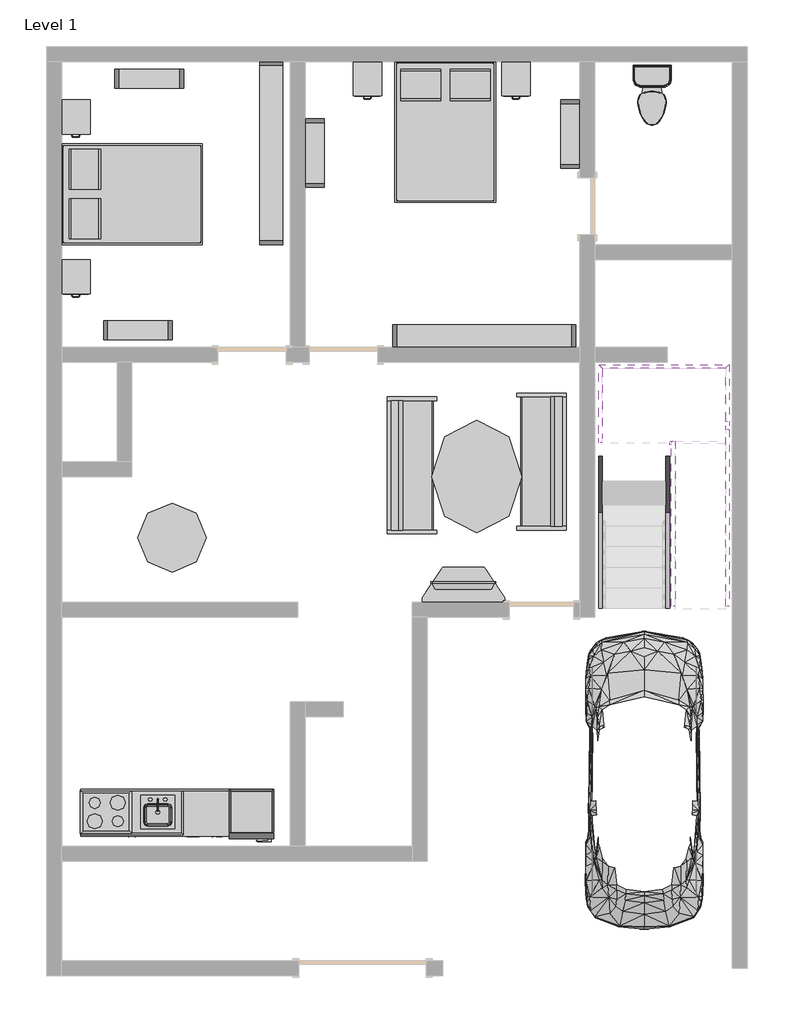
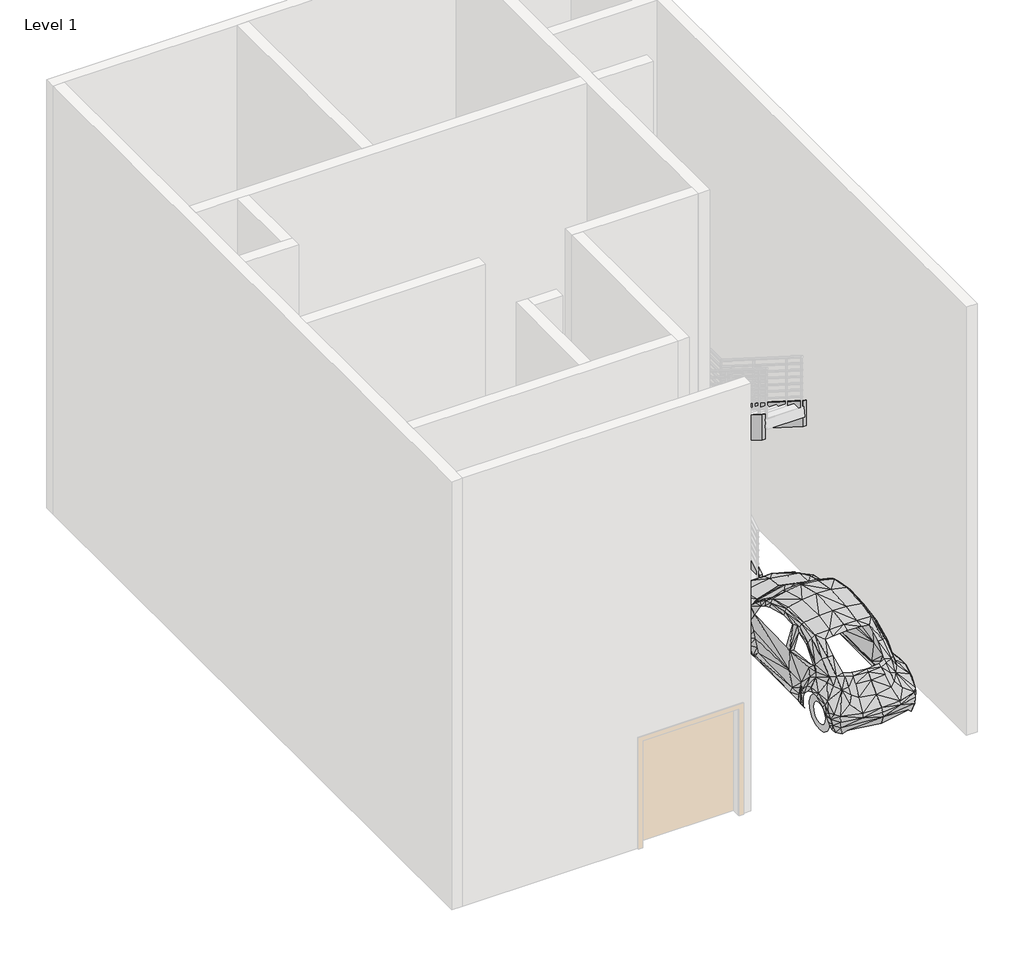
# One storey, part 4 of 4: 19 furniture elements, 8 members, 5 proxies, 2 flow terminals.
"""IFC4 building model written with IfcOpenShell, lengths in millimetres."""

from ifc_helpers import new_model, si_unit, frame, origin, place, context, project, spatial, polyline, outline, extrude, faceted_brep, transform, mapped, element, save
from components import m_cook_top_4_unit2_0615_x_500mm_249f3515, m_dishwasher_610_x_610_x_875mm_54ecfc4c, m_kitchenette_medium_1372mm_e05c6bec, m_rpc_beetle_m_rpc_beetle_b6d71803, m_refrigerator_600_x_660mm_a466bf94, m_sink_kitchen_island_450_x_450mm_f969cf2d, m_toilet_domestic_3d_m_toilet_domestic_3d_5cb52bd4, m_toilet_domestic_3d_m_toilet_domestic_3d_183bbd19, furniture_40ec15d9, furniture_0810mm_56245f3a, m_bed_box_1346_x_1880mm_double_b32eb57e, m_cabinet_file_2_drawer_0380_x_0457mm_9eec7cff, m_counter_top_w_sink_hole_600mm_depth_0a237b63, m_shelving_0915_x_0254_x_1830mm_1d5e155e, m_shelving_2440_x_0305_x_2134mm_59c1a9e4, m_sofa_1830mm_f9e8a66b, m_table_dining_round_w_chairs_0915mm_diameter_5defa876, m_table_ellipse_1500_x_1200mm_3917c766

model = new_model("IFC4")

# Units and contexts
model_context = context("Model", 3, world=origin())
ifc_project = project(units=[si_unit("LENGTHUNIT", "METRE", prefix="MILLI")], contexts=[model_context])

# Site, building, storey
site = spatial("IfcSite", under=ifc_project)
building = spatial("IfcBuilding", under=site)
storey = spatial("IfcBuildingStorey", under=building, Name="Level 1", Elevation=0.0)

# Proxies
placement = place(None, origin())
m_cook_top_4_unit2_0615_x_500mm_shape = m_cook_top_4_unit2_0615_x_500mm_249f3515(model_context)
element("IfcBuildingElementProxy", 1, Name="M_Cook Top-4 Unit2 : 0615 x 500mm", ObjectType="M_Cook Top-4 Unit2 : 0615 x 500mm", at=placement, inside=storey, context=model_context, shape_type="MappedRepresentation", body=[
    mapped(m_cook_top_4_unit2_0615_x_500mm_shape, transform((-6984.8389075, 2403.4805518, 0.0), x_axis=(1.0, 0.0, 0.0), y_axis=(0.0, 1.0, 0.0), z_axis=(0.0, 0.0, 1.0))),
])
m_dishwasher_610_x_610_x_875mm_shape = m_dishwasher_610_x_610_x_875mm_54ecfc4c(model_context)
element("IfcBuildingElementProxy", 2, Name="M_Dishwasher : 610 x 610 x 875mm", ObjectType="M_Dishwasher : 610 x 610 x 875mm", at=placement, inside=storey, context=model_context, shape_type="MappedRepresentation", body=[
    mapped(m_dishwasher_610_x_610_x_875mm_shape, transform((-6035.356376, 2136.830987, 0.0), x_axis=(1.0, 0.0, 0.0), y_axis=(0.0, 1.0, 0.0), z_axis=(0.0, 0.0, 1.0))),
])
m_kitchenette_medium_1372mm_shape = m_kitchenette_medium_1372mm_e05c6bec(model_context)
element("IfcBuildingElementProxy", 3, Name="M_Kitchenette - Medium : 1372mm", ObjectType="M_Kitchenette - Medium : 1372mm", at=placement, inside=storey, context=model_context, shape_type="MappedRepresentation", body=[
    mapped(m_kitchenette_medium_1372mm_shape, transform((-6660.5766124, 2708.4805518, 0.0), x_axis=(1.0, 0.0, 0.0), y_axis=(0.0, 1.0, 0.0), z_axis=(0.0, 0.0, 1.0))),
])
m_rpc_beetle_m_rpc_beetle_shape = m_rpc_beetle_m_rpc_beetle_b6d71803(model_context)
element("IfcBuildingElementProxy", 4, Name="M_RPC Beetle : M_RPC Beetle", ObjectType="M_RPC Beetle : M_RPC Beetle", at=placement, inside=storey, context=model_context, shape_type="MappedRepresentation", body=[
    mapped(m_rpc_beetle_m_rpc_beetle_shape, transform((192.3610925, 1592.0805518, 0.0), x_axis=(1.0, 0.0, 0.0), y_axis=(0.0, 1.0, 0.0), z_axis=(0.0, 0.0, 1.0))),
])
m_refrigerator_600_x_660mm_shape = m_refrigerator_600_x_660mm_a466bf94(model_context)
element("IfcBuildingElementProxy", 5, Name="M_Refrigerator : 600 x 660mm", ObjectType="M_Refrigerator : 600 x 660mm", at=placement, inside=storey, context=model_context, shape_type="MappedRepresentation", body=[
    mapped(m_refrigerator_600_x_660mm_shape, transform((-4994.0377648, 2412.2654616, 0.0), x_axis=(1.0, 0.0, 0.0), y_axis=(0.0, 1.0, 0.0), z_axis=(0.0, 0.0, 1.0))),
])

# Flow terminals
m_sink_kitchen_island_450_x_450mm_shape = m_sink_kitchen_island_450_x_450mm_f969cf2d(model_context)
element("IfcFlowTerminal", 6, ObjectType="M_Sink Kitchen-Island : 450 x 450mm", at=placement, inside=storey, context=model_context, shape_type="MappedRepresentation", body=[
    mapped(m_sink_kitchen_island_450_x_450mm_shape, transform((-6314.528148, 2401.1351507, 0.0), x_axis=(1.0, 0.0, 0.0), y_axis=(0.0, 1.0, 0.0), z_axis=(0.0, 0.0, 1.0))),
])
m_toilet_domestic_3d_m_toilet_domestic_3d_shape = m_toilet_domestic_3d_m_toilet_domestic_3d_5cb52bd4(model_context)
m_toilet_domestic_3d_m_toilet_domestic_3d_2_shape = m_toilet_domestic_3d_m_toilet_domestic_3d_183bbd19(model_context)
element("IfcFlowTerminal", 7, ObjectType="M_Toilet-Domestic-3D : M_Toilet-Domestic-3D", at=placement, inside=storey, context=model_context, shape_type="MappedRepresentation", body=[
    mapped(m_toilet_domestic_3d_m_toilet_domestic_3d_shape, transform((294.5650652, 11866.9845245, 0.0), x_axis=(1.0, 0.0, 0.0), y_axis=(0.0, 1.0, 0.0), z_axis=(0.0, 0.0, 1.0))),
    mapped(m_toilet_domestic_3d_m_toilet_domestic_3d_2_shape, transform((294.5650652, 11866.9845245, 0.0), x_axis=(1.0, 0.0, 0.0), y_axis=(0.0, 1.0, 0.0), z_axis=(0.0, 0.0, 1.0))),
])

# Furniture
furniture_shape = furniture_40ec15d9(model_context)
element("IfcFurniture", 8, at=placement, inside=storey, context=model_context, shape_type="MappedRepresentation", body=[
    mapped(furniture_shape, transform((-2345.8269095, 5670.4805518, 0.0), x_axis=(1.0, 0.0, 0.0), y_axis=(0.0, 1.0, 0.0), z_axis=(0.0, 0.0, 1.0))),
])
furniture_0810mm_shape = furniture_0810mm_56245f3a(model_context)
element("IfcFurniture", 9, ObjectType="0810mm", at=placement, inside=storey, context=model_context, shape_type="MappedRepresentation", body=[
    mapped(furniture_0810mm_shape, transform((-2224.5834216, 5406.0718602, 0.0), x_axis=(-1.0000000000000002, 0.0, 0.0), y_axis=(0.0, -1.0000000000000002, 0.0), z_axis=(0.0, 0.0, 1.0))),
])
m_bed_box_1346_x_1880mm_double_shape = m_bed_box_1346_x_1880mm_double_b32eb57e(model_context)
element("IfcFurniture", 10, ObjectType="M_Bed-Box : 1346 x 1880mm - Double", at=placement, inside=storey, context=model_context, shape_type="MappedRepresentation", body=[
    mapped(m_bed_box_1346_x_1880mm_double_shape, transform((-6876.0684157, 10306.3280928, 0.0), x_axis=(0.0, 1.0000000000000002, 0.0), y_axis=(-1.0000000000000002, 0.0, 0.0), z_axis=(0.0, 0.0, 1.0))),
])
element("IfcFurniture", 11, ObjectType="M_Bed-Box : 1346 x 1880mm - Double", at=placement, inside=storey, context=model_context, shape_type="MappedRepresentation", body=[
    mapped(m_bed_box_1346_x_1880mm_double_shape, transform((-2800.9913665, 11708.51006, 0.0), x_axis=(1.0000000000000009, 0.0, 0.0), y_axis=(0.0, 1.0000000000000009, 0.0), z_axis=(0.0, 0.0, 1.0))),
])
m_cabinet_file_2_drawer_0380_x_0457mm_shape = m_cabinet_file_2_drawer_0380_x_0457mm_9eec7cff(model_context)
element("IfcFurniture", 12, ObjectType="M_Cabinet-File 2 Drawer : 0380 x 0457mm", at=placement, inside=storey, context=model_context, shape_type="MappedRepresentation", body=[
    mapped(m_cabinet_file_2_drawer_0380_x_0457mm_shape, transform((-3374.9424604, 12327.7148519, 0.0), x_axis=(1.0, 0.0, 0.0), y_axis=(0.0, 1.0, 0.0), z_axis=(0.0, 0.0, 1.0))),
])
element("IfcFurniture", 13, ObjectType="M_Cabinet-File 2 Drawer : 0380 x 0457mm", at=placement, inside=storey, context=model_context, shape_type="MappedRepresentation", body=[
    mapped(m_cabinet_file_2_drawer_0380_x_0457mm_shape, transform((-1393.7424604, 12327.7148519, 0.0), x_axis=(1.0, 0.0, 0.0), y_axis=(0.0, 1.0, 0.0), z_axis=(0.0, 0.0, 1.0))),
])
element("IfcFurniture", 14, ObjectType="M_Cabinet-File 2 Drawer : 0380 x 0457mm", at=placement, inside=storey, context=model_context, shape_type="MappedRepresentation", body=[
    mapped(m_cabinet_file_2_drawer_0380_x_0457mm_shape, transform((-7263.7424604, 11818.1148519, 0.0), x_axis=(1.0, 0.0, 0.0), y_axis=(0.0, 1.0, 0.0), z_axis=(0.0, 0.0, 1.0))),
])
element("IfcFurniture", 15, ObjectType="M_Cabinet-File 2 Drawer : 0380 x 0457mm", at=placement, inside=storey, context=model_context, shape_type="MappedRepresentation", body=[
    mapped(m_cabinet_file_2_drawer_0380_x_0457mm_shape, transform((-7263.7424604, 9686.1148519, 0.0), x_axis=(1.0, 0.0, 0.0), y_axis=(0.0, 1.0, 0.0), z_axis=(0.0, 0.0, 1.0))),
])
m_counter_top_w_sink_hole_600mm_depth_shape = m_counter_top_w_sink_hole_600mm_depth_0a237b63(model_context)
element("IfcFurniture", 16, ObjectType="M_Counter Top w Sink Hole : 600mm Depth", at=placement, inside=storey, context=model_context, shape_type="MappedRepresentation", body=[
    mapped(m_counter_top_w_sink_hole_600mm_depth_shape, transform((-6127.3766124, 2708.4805518, 0.0), x_axis=(1.0, 0.0, 0.0), y_axis=(0.0, 1.0, 0.0), z_axis=(0.0, 0.0, 1.0))),
])
m_shelving_0915_x_0254_x_1830mm_shape = m_shelving_0915_x_0254_x_1830mm_1d5e155e(model_context)
element("IfcFurniture", 17, ObjectType="M_Shelving : 0915 x 0254 x 1830mm", at=placement, inside=storey, context=model_context, shape_type="MappedRepresentation", body=[
    mapped(m_shelving_0915_x_0254_x_1830mm_shape, transform((-6411.9389075, 12490.3805518, 0.0), x_axis=(1.0, 0.0, 0.0), y_axis=(0.0, 1.0, 0.0), z_axis=(0.0, 0.0, 1.0))),
])
element("IfcFurniture", 18, ObjectType="M_Shelving : 0915 x 0254 x 1830mm", at=placement, inside=storey, context=model_context, shape_type="MappedRepresentation", body=[
    mapped(m_shelving_0915_x_0254_x_1830mm_shape, transform((-6564.3389075, 9135.8805518, 0.0), x_axis=(1.0, 0.0, 0.0), y_axis=(0.0, 1.0, 0.0), z_axis=(0.0, 0.0, 1.0))),
])
element("IfcFurniture", 19, ObjectType="M_Shelving : 0915 x 0254 x 1830mm", at=placement, inside=storey, context=model_context, shape_type="MappedRepresentation", body=[
    mapped(m_shelving_0915_x_0254_x_1830mm_shape, transform((-4508.2389075, 11192.4805518, 0.0), x_axis=(0.0, 1.0, 0.0), y_axis=(-1.0, 0.0, 0.0), z_axis=(0.0, 0.0, 1.0))),
])
element("IfcFurniture", 20, ObjectType="M_Shelving : 0915 x 0254 x 1830mm", at=placement, inside=storey, context=model_context, shape_type="MappedRepresentation", body=[
    mapped(m_shelving_0915_x_0254_x_1830mm_shape, transform((-1101.4389075, 11446.9805518, 0.0), x_axis=(0.0, 1.0, 0.0), y_axis=(-1.0, 0.0, 0.0), z_axis=(0.0, 0.0, 1.0))),
])
m_shelving_2440_x_0305_x_2134mm_shape = m_shelving_2440_x_0305_x_2134mm_59c1a9e4(model_context)
element("IfcFurniture", 21, ObjectType="M_Shelving : 2440 x 0305 x 2134mm", at=placement, inside=storey, context=model_context, shape_type="MappedRepresentation", body=[
    mapped(m_shelving_2440_x_0305_x_2134mm_shape, transform((-1942.0389075, 9058.1805518, 0.0), x_axis=(1.0, 0.0, 0.0), y_axis=(0.0, 1.0, 0.0), z_axis=(0.0, 0.0, 1.0))),
])
element("IfcFurniture", 22, ObjectType="M_Shelving : 2440 x 0305 x 2134mm", at=placement, inside=storey, context=model_context, shape_type="MappedRepresentation", body=[
    mapped(m_shelving_2440_x_0305_x_2134mm_shape, transform((-5090.7389075, 11192.4805518, 0.0), x_axis=(0.0, 1.0000000000000002, 0.0), y_axis=(-1.0000000000000002, 0.0, 0.0), z_axis=(0.0, 0.0, 1.0))),
])
m_sofa_1830mm_shape = m_sofa_1830mm_f9e8a66b(model_context)
element("IfcFurniture", 23, ObjectType="M_Sofa : 1830mm", at=placement, inside=storey, context=model_context, shape_type="MappedRepresentation", body=[
    mapped(m_sofa_1830mm_shape, transform((-1325.3930058, 7147.2510436, 0.0), x_axis=(0.0, -1.0000000000000007, 0.0), y_axis=(1.0000000000000007, 0.0, 0.0), z_axis=(0.0, 0.0, 1.0))),
])
element("IfcFurniture", 24, ObjectType="M_Sofa : 1830mm", at=placement, inside=storey, context=model_context, shape_type="MappedRepresentation", body=[
    mapped(m_sofa_1830mm_shape, transform((-2758.6848091, 6957.31006, 0.0), x_axis=(0.0, 1.0000000000000002, 0.0), y_axis=(-1.0000000000000002, 0.0, 0.0), z_axis=(0.0, 0.0, 1.0))),
])
m_table_dining_round_w_chairs_0915mm_diameter_shape = m_table_dining_round_w_chairs_0915mm_diameter_5defa876(model_context)
element("IfcFurniture", 25, ObjectType="M_Table-Dining Round w Chairs : 0915mm Diameter", at=placement, inside=storey, context=model_context, shape_type="MappedRepresentation", body=[
    mapped(m_table_dining_round_w_chairs_0915mm_diameter_shape, transform((-6210.5208747, 6247.3592403, 0.0), x_axis=(1.0, 0.0, 0.0), y_axis=(0.0, 1.0, 0.0), z_axis=(0.0, 0.0, 1.0))),
])
m_table_ellipse_1500_x_1200mm_shape = m_table_ellipse_1500_x_1200mm_3917c766(model_context)
element("IfcFurniture", 26, ObjectType="M_Table-Ellipse : 1500 x 1200mm", at=placement, inside=storey, context=model_context, shape_type="MappedRepresentation", body=[
    mapped(m_table_ellipse_1500_x_1200mm_shape, transform((-2042.8389075, 6876.8805518, 0.0), x_axis=(0.0, 1.0, 0.0), y_axis=(-1.0, 0.0, 0.0), z_axis=(0.0, 0.0, 1.0))),
])

# Members
element("IfcMember", 27, ObjectType="Stringer - 50mm Width", at=placement, inside=storey, context=model_context, shape_type="SweptSolid", body=[
    extrude(outline(polyline([(5121.4805518, 0.0), (5121.4805518, 389.0025785), (7331.3115554, 1786.5241617), (7447.1806154, 1386.5241617), (5254.7392846, 0.0), (5121.4805518, 0.0)])), frame((-418.0389075, 0.0, 0.0), z_axis=(1.0, 0.0, 0.0), x_axis=(0.0, 1.0, 0.0)), (0.0, 0.0, 1.0), 50.0),
])
element("IfcMember", 28, ObjectType="Stringer - 50mm Width", at=placement, inside=storey, context=model_context, shape_type="SweptSolid", body=[
    extrude(outline(polyline([(5121.4805518, 0.0), (5121.4805518, 389.0025785), (7331.3115554, 1786.5241617), (7351.2805518, 1786.5241617), (7351.2805518, 1325.8759002), (5254.7392846, 0.0), (5121.4805518, 0.0)])), frame((479.5868738, 0.0, 0.0), z_axis=(1.0, 0.0, 0.0), x_axis=(0.0, 1.0, 0.0)), (0.0, 0.0, 1.0), 50.0),
])
element("IfcMember", 29, ObjectType="Stringer - 50mm Width", at=placement, inside=storey, context=model_context, shape_type="SweptSolid", body=[
    extrude(outline(polyline([(7616.4495483, 1786.5241617), (7500.5804883, 1386.5241617), (5151.2805518, 2872.2474417), (5151.2805518, 3345.5243176), (7616.4495483, 1786.5241617)])), frame((1275.5786001, 0.0, 0.0), z_axis=(1.0, 0.0, 0.0), x_axis=(0.0, 1.0, 0.0)), (0.0, 0.0, 1.0), 50.0),
])
element("IfcMember", 30, ObjectType="Stringer - 50mm Width", at=placement, inside=storey, context=model_context, shape_type="SweptSolid", body=[
    extrude(outline(polyline([(7351.2805518, 1954.2199698), (7351.2805518, 1480.9430939), (5151.2805518, 2872.2474417), (5151.2805518, 3345.5243176), (7351.2805518, 1954.2199698)])), frame((552.1868738, 0.0, 0.0), z_axis=(1.0, 0.0, 0.0), x_axis=(0.0, 1.0, 0.0)), (0.0, 0.0, 1.0), 50.0),
])
element("IfcMember", 31, ObjectType="Stringer - 50mm Width", at=placement, inside=storey, context=model_context, shape_type="Brep", body=[
    faceted_brep([(1275.5786001, 7616.4495483, 1786.5241617), (1325.5786001, 7616.4495483, 1786.5241617), (1325.5786001, 8371.5063331, 1786.5241617), (1275.5786001, 8321.5063331, 1786.5241617), (1275.5786001, 7500.5804883, 1386.5241617), (1275.5786001, 8321.5063331, 1386.5241617), (1325.5786001, 7500.5804883, 1386.5241617), (1325.5786001, 8371.5063331, 1386.5241617)], [[[0, 1, 2, 3]], [[4, 0, 3, 5]], [[6, 4, 5, 7]], [[1, 6, 7, 2]], [[1, 0, 4, 6]], [[2, 7, 5, 3]]]),
])
element("IfcMember", 32, ObjectType="Stringer - 50mm Width", at=placement, inside=storey, context=model_context, shape_type="SweptSolid", body=[
    extrude(outline(polyline([(1325.5786001, 8371.5063331), (1275.5786001, 8321.5063331), (-368.0389075, 8321.5063331), (-418.0389075, 8371.5063331), (1325.5786001, 8371.5063331)])), frame((0.0, 0.0, 1386.5241617), z_axis=(0.0, 0.0, 1.0), x_axis=(1.0, 0.0, 0.0)), (0.0, 0.0, 1.0), 400.0),
])
element("IfcMember", 33, ObjectType="Stringer - 50mm Width", at=placement, inside=storey, context=model_context, shape_type="Brep", body=[
    faceted_brep([(-368.0389075, 8321.5063331, 1786.5241617), (-418.0389075, 8371.5063331, 1786.5241617), (-418.0389075, 7331.3115554, 1786.5241617), (-368.0389075, 7331.3115554, 1786.5241617), (-368.0389075, 8321.5063331, 1386.5241617), (-368.0389075, 7447.1806154, 1386.5241617), (-418.0389075, 8371.5063331, 1386.5241617), (-418.0389075, 7447.1806154, 1386.5241617)], [[[0, 1, 2, 3]], [[4, 0, 3, 5]], [[6, 4, 5, 7]], [[1, 6, 7, 2]], [[1, 0, 4, 6]], [[2, 7, 5, 3]]]),
])
element("IfcMember", 34, ObjectType="Stringer - 50mm Width", at=placement, inside=storey, context=model_context, shape_type="SweptSolid", body=[
    extrude(outline(polyline([(529.5868738, 7301.2805518), (529.5868738, 7351.2805518), (552.1868738, 7351.2805518), (552.1868738, 7301.2805518), (529.5868738, 7301.2805518)])), frame((0.0, 0.0, 1386.5241617), z_axis=(0.0, 0.0, 1.0), x_axis=(1.0, 0.0, 0.0)), (0.0, 0.0, 1.0), 400.0),
])

save(model, "model.ifc")

# Revit data of these elements
# Type "M_Cook Top-4 Unit2 : 0615 x 500mm"
#   Depth = 500 mm
#   Width = 615 mm
#   Burner Material = Steel, Chrome Plated
#   Cooktop Material = Steel, Polished
#   Default Elevation = 0
#   Assembly Code = ""
# Type "M_Dishwasher : 610 x 610 x 875mm"
#   Label = "DW"
#   Depth = 610 mm
#   Height = 875 mm
#   Width = 610 mm
#   Dishwasher Material = Steel, Paint Finish, Ivory, Glossy
#   Panel Face Material = Plastic, Opaque Black
#   Default Elevation = 0
# Type "M_Kitchenette - Medium : 1372mm"
#   Counter Length = 1980 mm
#   Cabinet Width = 1372 mm
#   Cabinet Height = 900 mm
#   Cabinet Depth = 610 mm
#   Toe Depth = 35 mm
#   Toe Height = 100 mm
#   Cabinet Material = Cabinets
#   Door/Drawer Material = Cabinets
#   Handle Material = Cabinets - Handles
#   Default Elevation = 0
# Type "M_RPC Beetle : M_RPC Beetle"
#   built-in parameter 1005198 = "{2, 15},{39, RPC-16-0U6E-L4EG-ENH1-J3KF-SVEL-0TX4-C0},{1, 0},{1, 0},{2, 18},{1, 8},{5, Color},{1, 0},{1, 0},{3, 0.8},{3, 0.8},{3, 0.8},{1, 8},{7, BBoxMin},{1, 0},{1, 0},{1, 0},{1, 0},{1, 0},{1, 8},{7, BBoxMax},{1, 0},{1, 0},{1, 0},{1, 0},{1, 0},{2, 11},{9, RPCTypeId},{1, 0},{1, 0},{39, RPC-16-0U6E-L4EG-ENH1-J3KF-SVEL-0TX4-C0},{1, 6},{14, RPCPlantHeight},{1, 0},{1, 0},{4, 4.92},{2, 11},{7, keyword},{1, 0},{1, 0},{39, :RPCs:Auto_Economy/Midsize:Geometry:RPC},{2, 11},{8, category},{1, 0},{1, 0},{20, Auto_Economy/Midsize},{2, 11},{12, LocalizedUID},{1, 0},{1, 0},{13, VW Beetle [4]},{2, 14},{6, Height},{1, 0},{1, 0},{4, 4.92},{1, 2},{16, Cast Reflections},{1, 0},{1, 0},{1, 0},{1, 4},{12, Transparency},{1, 0},{1, 0},{2, 18},{1, 4},{7, Tinting},{1, 0},{1, 0},{2, 50},{1, 2},{11, Use Tinting},{1, 0},{1, 0},{1, 0},{1, 2},{13, License Plate},{1, 0},{1, 0},{1, 0},{2, 11},{21, License Plate Texture},{1, 0},{1, 0},{64, __RPC:/object data/textures/car/plate/textures/default/rgb/0/0/0},{2, 11},{23, i_License Plate Texture},{1, 0},{1, 0},{0, },{1, 2},{12, Custom Plate},{1, 0},{1, 0},{1, 0},{2, 11},{23, License Plate File Name},{1, 0},{1, 0},{0, },{21, assetlibrary_base.fbx},{1, 5},"
#   built-in parameter 1005195 = "RPC-16-0U6E-L4EG-ENH1-J3KF-SVEL-0TX4-C0"
#   Height = 0
# Type "M_Refrigerator : 600 x 660mm"
#   Label = "REF."
#   Depth = 660 mm
#   Height = 1830 mm
#   Width = 600 mm
#   Material = Steel, Paint Finish, Ivory, Matte
#   Description = (empty or 0)
#   Default Elevation = 0
# Type "M_Sink Kitchen-Island : 450 x 450mm"
#   Counter Height [instance default] = 900 mm
#   Depth = 450 mm
#   Width = 450 mm
#   Fixture Material = Steel, Polished
#   Sink Material = Steel, Polished
#   Default Elevation = 0
# Type "M_Toilet-Domestic-3D : M_Toilet-Domestic-3D"
#   Bowl/Basin Material = Porcelain, Linen
#   Seat Material = Laminate, Linen, Matte
#   Default Elevation = 0
# Type
#   Depth = 460 mm
#   Width = 1100 mm
#   Height = 500 mm
#   Finish = Melamine - Gray
#   Default Elevation = 0
# Type "0810mm"
#   SinAng = 0.49 mm
#   L = 705.961 mm
#   H = 397.139 mm
#   Thickness = 110 mm
#   Diagonal = 810 mm
#   CosAng = 0.872 mm
#   Stand [instance default] = yes
#   Default Elevation = 0
# Type "M_Bed-Box : 1346 x 1880mm - Double"
#   Length = 1880 mm
#   Width = 1346 mm
#   Frame Material = Birch
#   Mattress Material = Linen, White
#   Default Elevation = 0
# Type "M_Cabinet-File 2 Drawer : 0380 x 0457mm"
#   Depth = 457 mm
#   Height = 734 mm
#   Width = 380 mm
#   Cabinet Material = Steel, Paint Finish, Ivory, Glossy
#   Handle Material = Steel, Chrome Plated
#   Default Elevation = 0
# Type "M_Counter Top w Sink Hole : 600mm Depth"
#   Counter Thickness = 40 mm
#   Depth = 625 mm
#   Height = 900 mm
#   Length [instance default] = 2500 mm
#   Sink Location [instance default] = 1200 mm
#   Sink Location To Wall [instance default] = 100 mm
#   Sink Opening Depth [instance default] = 378 mm
#   Sink Opening Width [instance default] = 587 mm
#   Counter Top Material = none
#   Default Elevation = 0
# Type "M_Shelving : 0915 x 0254 x 1830mm"
#   Depth = 254 mm
#   Height = 1830 mm
#   Width = 915 mm
#   Material = Birch
#   Default Elevation = 0
# Type "M_Shelving : 2440 x 0305 x 2134mm"
#   Depth = 305 mm
#   Height = 2134 mm
#   Width = 2440 mm
#   Material = Laminate, Ivory, Matte
#   Default Elevation = 0
# Type "M_Sofa : 1830mm"
#   Width = 1830 mm
#   Seat Material = Linen, Beige
#   Frame Material = Cherry
#   Default Elevation = 0
# Type "M_Table-Dining Round w Chairs : 0915mm Diameter"
#   Radius = 457.5 mm
#   Diameter = 915 mm
#   Height = 762 mm
#   Chairs = 4
#   Base Material = Pine
#   Top Material = Laminate, Linen, Matte
#   Default Elevation = 0
# Type "M_Table-Ellipse : 1500 x 1200mm"
#   Half Width = 600 mm
#   Half Length = 750 mm
#   Height = 762 mm
#   Length = 1500 mm
#   Width = 1200 mm
#   Base Material = Birch
#   Top Material = Birch
#   Default Elevation = 0
#   Assembly Code = ""
# Element 1 (IfcBuildingElementProxy, "M_Cook Top-4 Unit2 : 0615 x 500mm")
#   Phase Created = New Construction
#   Materials on its faces: "Steel, Polished", "Steel, Chrome Plated"
# Element 2 (IfcBuildingElementProxy, "M_Dishwasher : 610 x 610 x 875mm")
#   Phase Created = New Construction
#   Materials on its faces: "Steel, Paint Finish, Ivory, Glossy", "Plastic, Opaque Black"
# Element 3 (IfcBuildingElementProxy, "M_Kitchenette - Medium : 1372mm")
#   Phase Created = New Construction
#   Materials on its faces: "Cabinets", "Cabinets - Handles"
# Element 4 (IfcBuildingElementProxy, "M_RPC Beetle : M_RPC Beetle")
#   Phase Created = New Construction
# Element 5 (IfcBuildingElementProxy, "M_Refrigerator : 600 x 660mm")
#   Phase Created = New Construction
#   Materials on its faces: "Steel, Paint Finish, Ivory, Matte", "Steel, Chrome Plated"
# Element 6 (IfcFlowTerminal, "M_Sink Kitchen-Island : 450 x 450mm")
#   Mark = "2"
#   Counter Height = 900 mm
#   Phase Created = New Construction
#   Materials on its faces: "Steel, Polished"
# Element 7 (IfcFlowTerminal, "M_Toilet-Domestic-3D : M_Toilet-Domestic-3D")
#   Mark = "1"
#   Phase Created = New Construction
#   Materials on its faces: "Porcelain, Linen", "Laminate, Linen, Matte"
# Element 8 (IfcFurniture)
#   Phase Created = New Construction
#   Materials on its faces: "Melamine - Gray", "Glass - Shelves"
# Element 9 (IfcFurniture, "0810mm")
#   Stand = yes
#   Phase Created = New Construction
#   Materials on its faces: "TV - Black", "TV - Glass", "TV - Screen"
# Elements 10, 11 (IfcFurniture, "M_Bed-Box : 1346 x 1880mm - Double")
#   Phase Created = New Construction
#   Materials on its faces: "Birch", "Linen, White"
# Elements 12, 13, 14, 15 (IfcFurniture, "M_Cabinet-File 2 Drawer : 0380 x 0457mm")
#   Phase Created = New Construction
#   Materials on its faces: "Steel, Chrome Plated", "Steel, Paint Finish, Ivory, Glossy"
# Element 16 (IfcFurniture, "M_Counter Top w Sink Hole : 600mm Depth")
#   Sink Opening Width = 400 mm
#   Sink Opening Depth = 350 mm
#   Sink Location To Wall = 160 mm
#   Sink Location = 1025 mm
#   Length = 1980 mm
#   Phase Created = New Construction
#   Materials on its faces: "Counter Top"
# Elements 17, 18, 19, 20 (IfcFurniture, "M_Shelving : 0915 x 0254 x 1830mm")
#   Phase Created = New Construction
#   Materials on its faces: "Birch"
# Elements 21, 22 (IfcFurniture, "M_Shelving : 2440 x 0305 x 2134mm")
#   Phase Created = New Construction
#   Materials on its faces: "Laminate, Ivory, Matte"
# Elements 23, 24 (IfcFurniture, "M_Sofa : 1830mm")
#   Phase Created = New Construction
#   Materials on its faces: "Cherry", "Linen, Beige"
# Element 25 (IfcFurniture, "M_Table-Dining Round w Chairs : 0915mm Diameter")
#   Phase Created = New Construction
#   Materials on its faces: "Pine", "Laminate, Linen, Matte"
# Element 26 (IfcFurniture, "M_Table-Ellipse : 1500 x 1200mm")
#   Phase Created = New Construction
#   Materials on its faces: "Birch"
# Elements 27, 28, 29, 30, 31, 32, 33, 34 (IfcMember, "Stringer - 50mm Width")
#   Phase Created = New Construction
# Materials
#   "Steel, Chrome Plated": class "Metal", colour RGB 244 244 244, transparency 0, Description = "Chromiuim plated steel", Cost = 0
#   "Steel, Polished": class "Metal", colour RGB 57 57 57, transparency 0, Description = "Polished steel", Cost = 0
#   "Steel, Paint Finish, Ivory, Glossy": class "Metal", colour RGB 247 247 239, transparency 0, Description = "Steel, paint finish, ivory, glossy", Cost = 0
#   "Plastic, Opaque Black": class "Plastic", colour RGB 0 0 0, transparency 0.7, Description = "Plastic, generic, opaque black", Cost = 0
#   "Cabinets": colour RGB 249 249 249, transparency 0
#   "Cabinets - Handles": class "Metal", colour RGB 57 57 57, transparency 0
#   "Steel, Paint Finish, Ivory, Matte": class "Metal", colour RGB 247 247 239, transparency 0, Description = "Steel, paint finish, ivory, matte", Cost = 0
#   "Porcelain, Linen": class "Ceramic", colour RGB 249 239 230, transparency 0, Description = "Porcelain, linen", Cost = 0
#   "Laminate, Linen, Matte": class "Plastic", colour RGB 249 239 230, transparency 0, Description = "Plastic Laminate - Linen, Matte", Cost = 0
#   "Melamine - Gray": class "Wood", colour RGB 49 49 49, transparency 0
#   "Birch": class "Wood", colour RGB 224 178 126, transparency 0, Description = "Betula Alleghaniensis", Cost = 0
#   "Linen, White": class "Textile", colour RGB 247 247 239, transparency 0, Description = "Linen, white", Cost = 0
#   "Laminate, Ivory, Matte": class "Plastic", colour RGB 247 247 229, transparency 0, Description = "Plastic Laminate - Ivory, Matte", Cost = 0
#   "Linen, Beige": class "Textile", colour RGB 249 239 230, transparency 0, Description = "Linen, beige", Cost = 0
#   "Cherry": class "Wood", colour RGB 154 107 61, transparency 0, Description = "Prunus Serotina", Cost = 0
#   "Pine": class "Wood", colour RGB 223 192 134, transparency 0, Description = "Pinus Echinata", Cost = 0
#   "Glass - Shelves": class "Glass", colour RGB 167 167 167, transparency 0.9
#   "TV - Black": colour RGB 49 49 49, transparency 0
#   "TV - Glass": colour RGB 157 157 157, transparency 0.9
#   "TV - Screen": colour RGB 0 0 0, transparency 0
#   "Counter Top": class "Wood", colour RGB 226 177 128, transparency 0
